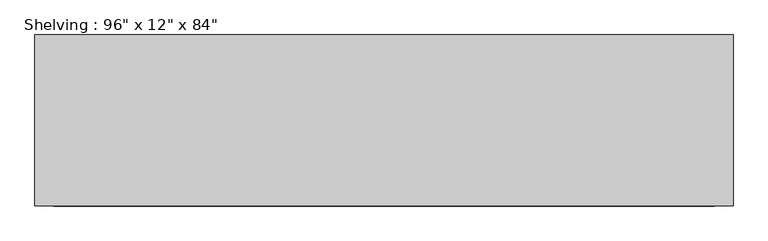
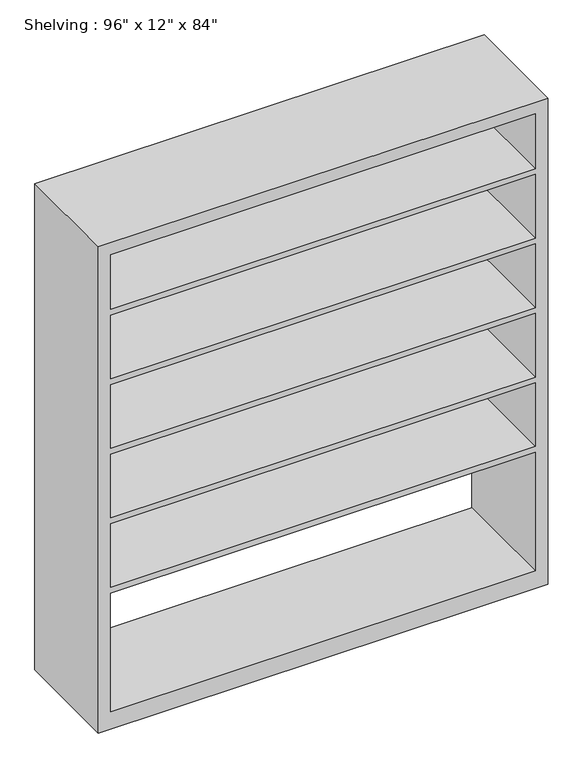
"""IFC4 building model written with IfcOpenShell, lengths in millimetres: furniture geometry."""

from ifc_helpers import new_model, si_unit, frame, origin, place, context, project, spatial, polyline, outline, extrude, source, transform, mapped, element, save


def furniture_53a00f75(model_context):
    return source(origin(), model_context, "Body", "SweptSolid", [
        extrude(outline(polyline([(0.0, 933.45), (2133.6, 933.45), (2133.6, -933.45), (0.0, -933.45), (0.0, 933.45)]), holes=[polyline([(2082.8, 882.65), (1841.5, 882.65), (1841.5, -882.65), (2082.8, -882.65), (2082.8, 882.65)]), polyline([(76.2, 882.65), (76.2, -882.65), (596.9, -882.65), (596.9, 882.65), (76.2, 882.65)]), polyline([(1231.9, -882.65), (1511.3, -882.65), (1511.3, 882.65), (1231.9, 882.65), (1231.9, -882.65)]), polyline([(1816.1, 882.65), (1536.7, 882.65), (1536.7, -882.65), (1816.1, -882.65), (1816.1, 882.65)]), polyline([(1206.5, 882.65), (927.1, 882.65), (927.1, -882.65), (1206.5, -882.65), (1206.5, 882.65)]), polyline([(901.7, 882.65), (622.3, 882.65), (622.3, -882.65), (901.7, -882.65), (901.7, 882.65)])]), frame((0.0, -533.4, 0.0), z_axis=(0.0, 1.0, 0.0), x_axis=(0.0, 0.0, 1.0)), (0.0, 0.0, 1.0), 457.2),
    ])


if __name__ == "__main__":
    model = new_model("IFC4")
    model_context = context("Model", 3, world=origin())
    ifc_project = project(units=[si_unit("LENGTHUNIT", "METRE", prefix="MILLI")], contexts=[model_context])
    site = spatial("IfcSite", under=ifc_project)
    building = spatial("IfcBuilding", under=site)
    placement = place(None, origin())
    furniture_shape = furniture_53a00f75(model_context)
    element("IfcFurniture", 1, ObjectType="Shelving : 96\" x 12\" x 84\"", at=placement, inside=building, context=model_context, shape_type="MappedRepresentation", body=[
        mapped(furniture_shape, transform((0.0, 0.0, 0.0), x_axis=(1.0, 0.0, 0.0), y_axis=(0.0, 1.0, 0.0), z_axis=(0.0, 0.0, 1.0))),
    ])
    save(model, "model.ifc")

# Revit data of these elements
# Type "Shelving : 96\" x 12\" x 84\""
#   Assembly Code = "E2020200"
#   Depth = 1' - 6"
#   Height = 7' - 0"
#   Width = 6' - 1 1/2"
#   Shelving Unit Material = Laminate, Ivory, Matte
#   Default Elevation = 0
# Element 1 (IfcFurniture, "Shelving : 96\" x 12\" x 84\"")
#   Materials on its faces: "Laminate, Ivory, Matte"
# Materials
#   "Laminate, Ivory, Matte": class "Plastic", colour RGB 247 247 239, transparency 0, Description = "Plastic Laminate - Ivory, Matte", Cost = 0
